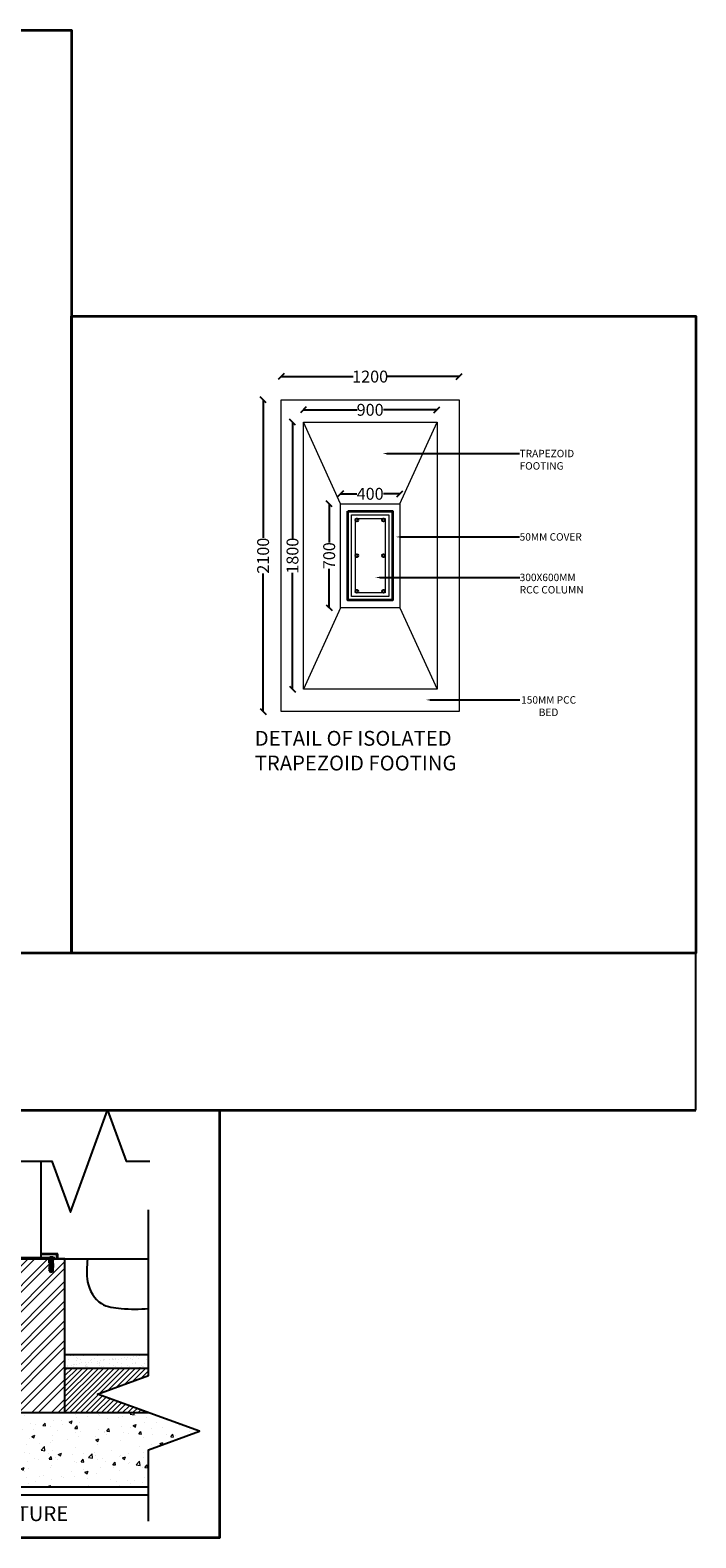
# Model space of a CAD drawing. Units: millimetres. Extents: x -6233 to 6805, y -5269 to 4890.
# Tile 4 of 4: x 2321 to 6805, y -5269 to 4890. Entities that reach past the tile are written whole.
import ezdxf
from ezdxf import colors
from ezdxf.entities.mleader import LeaderData, LeaderLine
from ezdxf.math import Vec2, Vec3

# ---------------------------------------------------------------- set-up
doc = ezdxf.new("R2010")
doc.units = ezdxf.units.MM
doc.header["$MEASUREMENT"] = 0
for name, color, linetype, lineweight in [('A-FLOR-HRAL', 4, 'Continuous', 25), ('S-ANNO-DIMS', 2, 'Continuous', 18), ('S-ANNO-TEXT', 3, 'Continuous', 18), ('S-ANNO-TTLB', 7, 'Continuous', 35), ('S-CONC', 7, 'Continuous', 35), ('S-FNDN', 8, 'Continuous', 18), ('S-PATT', 252, 'Continuous', 13), ('S-REIN', 1, 'Continuous', 25)]:
    doc.layers.add(name, color=color, linetype=linetype, lineweight=lineweight)
doc.styles.get("Standard").update_dxf_attribs({"font": 'arial.ttf'})
doc.dimstyles.get("Standard").update_dxf_attribs({"dimtxt": 80, "dimasz": 40, "dimexe": 0.18, "dimexo": 0.0625, "dimgap": 0.09, "dimtad": 0, "dimdec": 0, "dimzin": 0, "dimdsep": 46, "dimtxsty": 'Standard', "dimblk": 'OBLIQUE', "dimcen": 0.09, "dimadec": 0, "dimazin": 0, "dimtfac": 1, "dimtdec": 0, "dimtofl": 0, "dimtmove": 0, "dimatfit": 3, "dimfxl": 1, "dimfxlon": 1, "dimtolj": 1, "dimtzin": 0, "dimarcsym": 0})

# ---------------------------------------------------------------- blocks, each defined once
blk = doc.blocks.new('_Oblique')
at = {"color": 0, "linetype": 'ByBlock', "lineweight": -2}
blk.add_line((-0.5, -0.5), (0.5, 0.5), dxfattribs=at)
blk = doc.blocks.new('*D17')
at = {"layer": 'DEFPOINTS', "color": 0, "transparency": 16777216}
for p in [(4011, 2556), (4011, 2399), (5211, 2399)]:
    blk.add_point(p, dxfattribs=at)
at = {"layer": 'S-ANNO-DIMS', "color": 0, "lineweight": -2, "transparency": 16777216}
for p, q in [((4011, 2555), (4011, 2556)), ((4011, 2556), (4496, 2556)), ((5211, 2556), (4727, 2556)), ((5211, 2555), (5211, 2556))]:
    blk.add_line(p, q, dxfattribs=at)
at = {"layer": 'S-ANNO-DIMS', "color": 0, "lineweight": -2, "transparency": 16777216, "xscale": 40, "yscale": 40, "zscale": 40, "rotation": 180}
blk.add_blockref('_Oblique', (4011, 2556), dxfattribs=at)
at = {"layer": 'S-ANNO-DIMS', "color": 0, "lineweight": -2, "transparency": 16777216, "xscale": 40, "yscale": 40, "zscale": 40}
blk.add_blockref('_Oblique', (5211, 2556), dxfattribs=at)
at = {"layer": 'S-ANNO-DIMS', "color": 0, "transparency": 16777216, "insert": (4611, 2556), "char_height": 80, "attachment_point": 5}
blk.add_mtext('\\A1;1200', dxfattribs=at)
blk = doc.blocks.new('*D18')
at = {"layer": 'DEFPOINTS', "color": 0, "transparency": 16777216}
for p in [(4011, 2399), (3890, 299), (4011, 299)]:
    blk.add_point(p, dxfattribs=at)
at = {"layer": 'S-ANNO-DIMS', "color": 0, "lineweight": -2, "transparency": 16777216}
for p, q in [((3891, 2399), (3890, 2399)), ((3890, 2399), (3890, 1469)), ((3890, 299), (3890, 1229)), ((3891, 299), (3890, 299))]:
    blk.add_line(p, q, dxfattribs=at)
at = {"layer": 'S-ANNO-DIMS', "color": 0, "lineweight": -2, "transparency": 16777216, "xscale": 40, "yscale": 40, "zscale": 40}
for p, rotation in [((3890, 2399), 90), ((3890, 299), 270)]:
    blk.add_blockref('_Oblique', p, dxfattribs=dict(at, rotation=rotation))
at = {"layer": 'S-ANNO-DIMS', "color": 0, "transparency": 16777216, "insert": (3890, 1349), "char_height": 80, "attachment_point": 5, "rotation": 90}
blk.add_mtext('\\A1;2100', dxfattribs=at)
blk = doc.blocks.new('*D19')
at = {"layer": 'DEFPOINTS', "color": 0, "transparency": 16777216}
for p in [(4161, 2332), (4161, 2249), (5061, 2249)]:
    blk.add_point(p, dxfattribs=at)
at = {"layer": 'S-ANNO-DIMS', "color": 0, "lineweight": -2, "transparency": 16777216}
for p, q in [((4161, 2331), (4161, 2332)), ((4161, 2332), (4523, 2332)), ((5061, 2332), (4700, 2332)), ((5061, 2331), (5061, 2332))]:
    blk.add_line(p, q, dxfattribs=at)
at = {"layer": 'S-ANNO-DIMS', "color": 0, "lineweight": -2, "transparency": 16777216, "xscale": 40, "yscale": 40, "zscale": 40, "rotation": 180}
blk.add_blockref('_Oblique', (4161, 2332), dxfattribs=at)
at = {"layer": 'S-ANNO-DIMS', "color": 0, "lineweight": -2, "transparency": 16777216, "xscale": 40, "yscale": 40, "zscale": 40}
blk.add_blockref('_Oblique', (5061, 2332), dxfattribs=at)
at = {"layer": 'S-ANNO-DIMS', "color": 0, "transparency": 16777216, "insert": (4611, 2332), "char_height": 80, "attachment_point": 5}
blk.add_mtext('\\A1;900', dxfattribs=at)
blk = doc.blocks.new('*D20')
at = {"layer": 'DEFPOINTS', "color": 0, "transparency": 16777216}
for p in [(4161, 2249), (4088, 449), (4161, 449)]:
    blk.add_point(p, dxfattribs=at)
at = {"layer": 'S-ANNO-DIMS', "color": 0, "lineweight": -2, "transparency": 16777216}
for p, q in [((4089, 2249), (4087, 2249)), ((4088, 2249), (4088, 1464)), ((4088, 449), (4088, 1233)), ((4089, 449), (4087, 449))]:
    blk.add_line(p, q, dxfattribs=at)
at = {"layer": 'S-ANNO-DIMS', "color": 0, "lineweight": -2, "transparency": 16777216, "xscale": 40, "yscale": 40, "zscale": 40}
for p, rotation in [((4088, 2249), 90), ((4088, 449), 270)]:
    blk.add_blockref('_Oblique', p, dxfattribs=dict(at, rotation=rotation))
at = {"layer": 'S-ANNO-DIMS', "color": 0, "transparency": 16777216, "insert": (4088, 1349), "char_height": 80, "attachment_point": 5, "rotation": 90}
blk.add_mtext('\\A1;1800', dxfattribs=at)
blk = doc.blocks.new('*D21')
at = {"layer": 'DEFPOINTS', "color": 0, "transparency": 16777216}
for p in [(4811, 1766), (4411, 1699), (4811, 1699)]:
    blk.add_point(p, dxfattribs=at)
at = {"layer": 'S-ANNO-DIMS', "color": 0, "lineweight": -2, "transparency": 16777216}
for p, q in [((4411, 1765), (4411, 1766)), ((4411, 1766), (4521, 1766)), ((4811, 1766), (4701, 1766)), ((4811, 1765), (4811, 1766))]:
    blk.add_line(p, q, dxfattribs=at)
at = {"layer": 'S-ANNO-DIMS', "color": 0, "lineweight": -2, "transparency": 16777216, "xscale": 40, "yscale": 40, "zscale": 40, "rotation": 180}
blk.add_blockref('_Oblique', (4411, 1766), dxfattribs=at)
at = {"layer": 'S-ANNO-DIMS', "color": 0, "lineweight": -2, "transparency": 16777216, "xscale": 40, "yscale": 40, "zscale": 40}
blk.add_blockref('_Oblique', (4811, 1766), dxfattribs=at)
at = {"layer": 'S-ANNO-DIMS', "color": 0, "transparency": 16777216, "insert": (4611, 1766), "char_height": 80, "attachment_point": 5}
blk.add_mtext('\\A1;400', dxfattribs=at)
blk = doc.blocks.new('*D22')
at = {"layer": 'DEFPOINTS', "color": 0, "transparency": 16777216}
for p in [(4411, 1699), (4335, 999), (4411, 999)]:
    blk.add_point(p, dxfattribs=at)
at = {"layer": 'S-ANNO-DIMS', "color": 0, "lineweight": -2, "transparency": 16777216}
for p, q in [((4336, 1699), (4335, 1699)), ((4335, 1699), (4335, 1437)), ((4335, 999), (4335, 1261)), ((4336, 999), (4335, 999))]:
    blk.add_line(p, q, dxfattribs=at)
at = {"layer": 'S-ANNO-DIMS', "color": 0, "lineweight": -2, "transparency": 16777216, "xscale": 40, "yscale": 40, "zscale": 40}
for p, rotation in [((4335, 1699), 90), ((4335, 999), 270)]:
    blk.add_blockref('_Oblique', p, dxfattribs=dict(at, rotation=rotation))
at = {"layer": 'S-ANNO-DIMS', "color": 0, "transparency": 16777216, "insert": (4335, 1349), "char_height": 80, "attachment_point": 5, "rotation": 90}
blk.add_mtext('\\A1;700', dxfattribs=at)

msp = doc.modelspace()

# ---------------------------------------------------------------- hatches: boundary and pattern name
at = {"layer": 'S-PATT'}
h = msp.add_hatch(dxfattribs=at)
h.set_pattern_fill('ANSI32', color=256, scale=250)
h.set_pattern_definition([(45, (-403.88, 395.55), (-66.2913, 66.2913), []), (45, (-359.68, 395.55), (-66.2913, 66.2913), [])])
h.paths.add_polyline_path([(2555.6, -3388.6), (2479.2, -3388.6), (2475, -3412), (2479.2, -3425.9), (2479.2, -3442.8), (2477.2, -3451.1), (2477.2, -3475.2), (2457.7, -3479.6), (2450.6, -3467.1), (2447.4, -3461.6), (2448.4, -3451.9), (2451.4, -3421.4), (2447.5, -3414.8), (2447.5, -3401.8), (2448.7, -3388.6), (2096.7, -3388.6), (2092.6, -3412), (2096.7, -3425.9), (2096.7, -3442.8), (2094.8, -3451), (2094.8, -3475.2), (2075.3, -3479.6), (2068.2, -3467.1), (2065, -3461.6), (2065.9, -3451.9), (2069, -3421.4), (2065.1, -3414.8), (2065.1, -3401.8), (2066.2, -3388.6), (1993.8, -3388.6), (1993.8, -4425), (2555.6, -4425)])
h = msp.add_hatch(dxfattribs=at)
h.set_pattern_fill('AR-SAND', color=256, scale=30)
h.set_pattern_definition([(37.5, (-403.876, 395.554), (-1.8898, 57.8047), [0, -45.6, 0, -51, 0, -48.75]), (7.5, (-403.88, 395.554), (53.0933, 84.6644), [0, -24.6, 0, -41.1, 0, -15.75]), (327.5, (-440.776, 395.554), (93.42426, 0.16977), [0, -15, 0, -54, 0, -70.5]), (317.5, (-440.78, 395.55), (90.1838, 26.3303), [0, -7.5, 0, -35.4, 0, -40.5])])
h.paths.add_polyline_path([(2555.6, -4032.9), (2555.6, -4125), (3117.4, -4125), (3117.4, -4032.9)])
h = msp.add_hatch(dxfattribs=at)
h.set_pattern_fill('ANSI31', color=256, scale=200)
h.set_pattern_definition([(45, (-403.876, 395.554), (-17.67767, 17.67767), [])])
h.paths.add_polyline_path([(2555.6, -4125), (2555.6, -4425), (3117.4, -4425), (2773.9, -4300), (3117.4, -4175), (3117.4, -4125)])
h = msp.add_hatch(dxfattribs=at)
h.set_pattern_fill('AR-CONC', color=256, scale=30)
h.set_pattern_definition([(50, (-403.88, 395.55), (215.178, -18.8256), [22.5, -247.5]), (355, (-403.88, 395.55), (-41.6254, 225.658), [18, -198]), (100.4514, (-385.94, 393.99), (173.5527, 206.832), [19.122, -210.3426]), (46.184, (-403.88, 455.55), (320.172, -49.656), [33.75, -371.25]), (96.6356, (-377.2, 451.42), (280.399, 292.236), [28.683, -315.514]), (351.184, (-403.88, 455.55), (280.399, 292.236), [27, -297]), (21, (-373.88, 440.55), (179.072, -120.7857), [22.5, -247.5]), (326, (-373.88, 440.55), (72.9946, 217.545), [18, -198]), (71.4514, (-358.95, 430.49), (252.067, 96.7593), [19.122, -210.3426]), (37.5, (-403.88, 395.554), (3.648, 99.8682), [0, -195.6, 0, -201, 0, -198.75]), (7.5, (-403.88, 395.55), (78.9209, 118.3235), [0, -114.6, 0, -191.1, 0, -75.75]), (327.5, (-470.78, 395.55), (160.1467, -6.7665), [0, -75, 0, -234, 0, -310.5]), (317.5, (-500.78, 395.55), (174.9559, 30.0315), [0, -97.5, 0, -155.4, 0, -220.5])])
h.paths.add_polyline_path([(3117.4, -4925), (3117.4, -4675), (3460.8, -4550), (3117.4, -4425), (1993.8, -4425), (1993.8, -4925)])

# ---------------------------------------------------------------- linework, layer by layer
at = {"layer": 'A-FLOR-HRAL'}
for p, q in [((6804.5, -2387.1), (6804.5, -1330.2)), ((2395.6, -3388.6), (2395.6, -2730.5)), ((2486.4, -3382.1), (2057.2, -3382.1)), ((2089.6, -3388.6), (2459.7, -3388.6)), ((2459.7, -3388.6), (2089.6, -3388.6)), ((2507, -3355.2), (2395.6, -3355.2)), ((2501.1, -3359.8), (2395.6, -3359.8)), ((2448.4, -3451.9), (2447.4, -3461.6)), ((2448.7, -3388.6), (2447.5, -3401.8)), ((2447.5, -3401.8), (2447.5, -3414.8)), ((2447.5, -3414.8), (2451.4, -3421.4)), ((2451.4, -3421.4), (2448.4, -3451.9)), ((2454.6, -3382.1), (2454.6, -3376)), ((2454.6, -3376), (2477.1, -3376)), ((2460.9, -3382.1), (2454.6, -3382.1)), ((2459.7, -3472.8), (2459.7, -3382.1)), ((2460.9, -3382.1), (2473.3, -3382.1)), ((2472.1, -3382.1), (2472.1, -3472.8)), ((2555.6, -3388.6), (2472.1, -3388.6)), ((2472.1, -3388.6), (3117.4, -3388.6)), ((2477.1, -3382.1), (2473.3, -3382.1)), ((2475, -3412), (2479.2, -3388.6)), ((2479.2, -3425.9), (2475, -3412)), ((2477.1, -3376), (2477.1, -3382.1)), ((2477.2, -3450), (2479.2, -3442.8)), ((2477.2, -3475.2), (2477.2, -3450)), ((2479.2, -3442.8), (2479.2, -3425.9)), ((2486.4, -3388.6), (2486.4, -3382.1)), ((2501.1, -3388.6), (2501.1, -3359.8)), ((2507, -3388.6), (2507, -3355.2)), ((2555.6, -4425), (2555.6, -3388.6)), ((2447.4, -3461.6), (2450.6, -3467.1)), ((2450.6, -3467.1), (2457.7, -3479.6)), ((2457.7, -3479.6), (2477.2, -3475.2)), ((2472.1, -3472.8), (2459.7, -3472.8)), ((2555.6, -4032.9), (3117.4, -4032.9)), ((2555.6, -4125), (3117.4, -4125)), ((1993.8, -4425), (3117.4, -4425)), ((1993.8, -4925), (3117.4, -4925)), ((1943.8, -4979.4), (3117.4, -4979.4))]:
    msp.add_line(p, q, dxfattribs=at)
for points in [[(1954.9, -2730.5), (2467.4, -2730.5), (2592.4, -3073.9), (2842.4, -2387.1), (2967.4, -2730.5), (3126.4, -2730.5)], [(3117.4, -5156.4), (3117.4, -4675), (3460.8, -4550), (2773.9, -4300), (3117.4, -4175), (3117.4, -3059.1)]]:
    msp.add_lwpolyline(points, dxfattribs=at)
msp.add_open_spline([(2708.2, -3388.6), (2702.7, -3440.4), (2691.1, -3549.8), (2778.8, -3706.5), (2951.5, -3727.5), (3057.2, -3729.7), (3117.4, -3723.4)], degree=3, knots=[0, 0, 0, 0, 155.578029, 328.7299587, 465.7286102, 648.9577579, 648.9577579, 648.9577579, 648.9577579], dxfattribs=at)
at = {"layer": 'S-ANNO-TTLB'}
msp.add_line((-6232.9, -2387.1), (6804.5, -2387.1), dxfattribs=at)
for points in [[(-6232.9, 4890.2), (2600.5, 4890.2), (2600.5, -1330.2), (-6232.9, -1330.2)], [(2600.5, 2963.4), (6804.5, 2963.4), (6804.5, -1330.2), (2600.5, -1330.2)], [(499.3, -2387.1), (3596.8, -2387.1), (3596.8, -5268.9), (499.3, -5268.9)]]:
    msp.add_lwpolyline(points, close=True, dxfattribs=at)
at = {"layer": 'S-CONC'}
msp.add_lwpolyline([(4461.3, 1648.7), (4761.3, 1648.7), (4761.3, 1048.7), (4461.3, 1048.7)], close=True, dxfattribs=at)
at = {"layer": 'S-FNDN'}
for p, q in [((4411.3, 1698.7), (4161.3, 2248.7)), ((4811.3, 1698.7), (5061.3, 2248.7)), ((4411.3, 998.7), (4161.3, 448.7)), ((4811.3, 998.7), (5061.3, 448.7))]:
    msp.add_line(p, q, dxfattribs=at)
for points in [[(4011.3, 2398.7), (5211.3, 2398.7), (5211.3, 298.7), (4011.3, 298.7)], [(4161.3, 2248.7), (5061.3, 2248.7), (5061.3, 448.7), (4161.3, 448.7)], [(4411.3, 1698.7), (4811.3, 1698.7), (4811.3, 998.7), (4411.3, 998.7)], [(4486.3, 1623.7), (4736.3, 1623.7), (4736.3, 1073.7), (4486.3, 1073.7)], [(4511.3, 1598.7), (4711.3, 1598.7), (4711.3, 1098.7), (4511.3, 1098.7)]]:
    msp.add_lwpolyline(points, close=True, dxfattribs=at)
at = {"layer": 'S-REIN'}
for centre in [(4521.1, 1588.9), (4701.5, 1588.9), (4521.1, 1349.7), (4701.5, 1349.7), (4521.1, 1108.5), (4701.5, 1108.5)]:
    msp.add_circle(centre, 9.8, dxfattribs=at)

# ---------------------------------------------------------------- texts
at = {"layer": 'S-ANNO-TEXT', "char_height": 100, "attachment_point": 1}
for s, width, insert in [('DETAIL OF ISOLATED\\PTRAPEZOID FOOTING', 1812.356, (3833.9, 168.5)), ('BALCONY RAILING FIXTURE', 2161.186, (853.7, -5055.9))]:
    msp.add_mtext_dynamic_manual_height_columns(s, width=width, gutter_width=1, heights=[0], dxfattribs=dict(at, insert=insert))

# ---------------------------------------------------------------- dimensions: what is measured, and where the dimension line sits
at = {"layer": 'S-ANNO-DIMS'}
for base, p1, p2, picture, middle in [((4011.3, 2555.6), (5211.3, 2398.7), (4011.3, 2398.7), '*D17', (4611.3, 2555.6)), ((4161.3, 2331.9), (5061.3, 2248.7), (4161.3, 2248.7), '*D19', (4611.3, 2331.9)), ((4811.3, 1766.1), (4411.3, 1698.7), (4811.3, 1698.7), '*D21', (4611.3, 1766.1))]:
    dim = msp.add_linear_dim(base=base, p1=p1, p2=p2, dimstyle='Standard', override={"dimclrd": 0, "dimclre": 0, "dimclrt": 0}, dxfattribs=at)
    dim.commit()
    dim.dimension.update_dxf_attribs({"geometry": picture, "text_midpoint": middle})
for base, p1, p2, picture, middle in [((3889.9, 298.7), (4011.3, 2398.7), (4011.3, 298.7), '*D18', (3889.9, 1348.7)), ((4087.7, 448.7), (4161.3, 2248.7), (4161.3, 448.7), '*D20', (4087.7, 1348.7)), ((4334.7, 998.7), (4411.3, 1698.7), (4411.3, 998.7), '*D22', (4334.7, 1348.7))]:
    dim = msp.add_linear_dim(base=base, p1=p1, p2=p2, angle=90, dimstyle='Standard', override={"dimclrd": 0, "dimclre": 0, "dimclrt": 0}, dxfattribs=at)
    dim.commit()
    dim.dimension.update_dxf_attribs({"geometry": picture, "text_midpoint": middle})

# ---------------------------------------------------------------- leaders
at = {"layer": 'S-ANNO-TEXT'}
ml = msp.add_multileader_mtext('Standard', dxfattribs=at)
ml.set_content('TRAPEZOID\\PFOOTING', color=256)
ml.set_leader_properties()
ml.build(insert=Vec2(0, 0))
ml.multileader.update_dxf_attribs({"dogleg_length": 0.36, "arrow_head_size": 30})
ctx = ml.context
ctx.base_point, ctx.char_height, ctx.arrow_head_size, ctx.landing_gap_size, ctx.plane_origin = Vec3(5617.4, 2037), 50, 30, 0.09, Vec3(4693.9, 2037)
notes = []
notes.append((ctx, [(0, (1, 1, 0), (5617.1, 2037), (1, 0), 0.36, [(0, [(4693.9, 2037)], 0, [])])]))
ctx.mtext.insert, ctx.mtext.flow_direction = Vec3(5617.5, 2062.4), 5
ml = msp.add_multileader_mtext('Standard', dxfattribs=at)
ml.set_content('50MM COVER', color=256)
ml.set_leader_properties()
ml.build(insert=Vec2(0, 0))
ml.multileader.update_dxf_attribs({"dogleg_length": 0.36, "arrow_head_size": 30})
ctx = ml.context
ctx.base_point, ctx.char_height, ctx.arrow_head_size, ctx.landing_gap_size, ctx.plane_origin = Vec3(5617.8, 1475.3), 50, 30, 0.09, Vec3(4782.8, 1475.3)
notes.append((ctx, [(0, (1, 1, 0), (5617.4, 1475.3), (1, 0), 0.36, [(0, [(4782.8, 1475.3)], 0, [])])]))
ctx.mtext.insert, ctx.mtext.flow_direction = Vec3(5617.9, 1500.7), 5
ml = msp.add_multileader_mtext('Standard', dxfattribs=at)
ml.set_content('{\\C256;300X600MM\\PRCC COLUMN}', color=256)
ml.set_leader_properties()
ml.build(insert=Vec2(0, 0))
ml.multileader.update_dxf_attribs({"dogleg_length": 0.36, "arrow_head_size": 30})
ctx = ml.context
ctx.base_point, ctx.char_height, ctx.arrow_head_size, ctx.landing_gap_size, ctx.plane_origin = Vec3(5618.1, 1202.3), 50, 30, 0.09, Vec3(4645.2, 1202.3)
notes.append((ctx, [(0, (1, 1, 0), (5617.8, 1202.3), (1, 0), 0.36, [(0, [(4645.2, 1202.3)], 0, [])])]))
ctx.mtext.insert, ctx.mtext.flow_direction = Vec3(5618.2, 1227.7), 5
ml = msp.add_multileader_mtext('Standard', dxfattribs=at)
ml.set_content('150MM PCC\\PBED', color=256)
ml.set_leader_properties()
ml.build(insert=Vec2(0, 0))
ml.multileader.update_dxf_attribs({"dogleg_length": 0.36, "arrow_head_size": 30})
ctx = ml.context
ctx.base_point, ctx.char_height, ctx.arrow_head_size, ctx.landing_gap_size, ctx.plane_origin = Vec3(5618.1, 377.2), 50, 30, 0.09, Vec3(4985.9, 377.2)
ctx.text_align_type = 1
notes.append((ctx, [(0, (1, 1, 0), (5617.8, 377.2), (1, 0), 0.36, [(0, [(4985.9, 377.2)], 0, [])])]))
ctx.mtext.insert, ctx.mtext.alignment, ctx.mtext.flow_direction = Vec3(5812.9, 402.2), 2, 5
for ctx, leaders in notes:
    for number, flags, end, landing, length, lines in leaders:
        leader = LeaderData()
        leader.index, (leader.has_last_leader_line, leader.has_dogleg_vector, leader.attachment_direction) = number, flags
        leader.last_leader_point, leader.dogleg_vector, leader.dogleg_length = Vec3(end), Vec3(landing), length
        for number, points, colour, breaks in lines:
            line = LeaderLine()
            line.index, line.vertices, line.color, line.breaks = number, Vec3.list(points), colors.encode_raw_color(colour), breaks
            leader.lines.append(line)
        ctx.leaders.append(leader)

doc.saveas('drawing.dxf')
